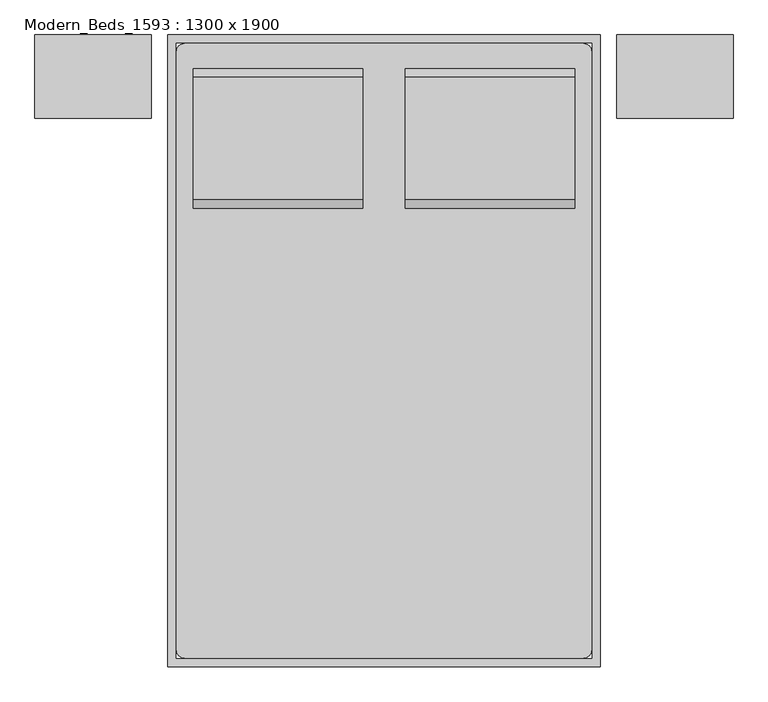
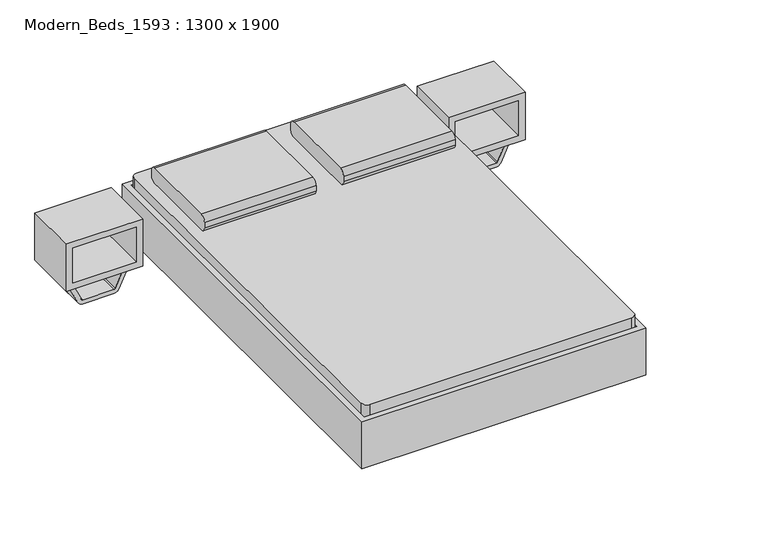
"""IFC4 building model written with IfcOpenShell, lengths in millimetres: furniture geometry, Modern_Beds_1593 : 1300 x 1900."""

from ifc_helpers import new_model, si_unit, point, frame, frame_2d, origin, place, context, project, spatial, polyline, circle_curve, trimmed, segment, composite_curve, outline, extrude, source, transform, mapped, element, save
from ifc_brep_helpers import plane_surface, cylinder_surface, revolved_surface, advanced_brep


def modern_beds_1593_1300_x_1900_cc95cf5d(model_context):
    return source(origin(), model_context, "Body", "SolidModel", [
        advanced_brep(
        [(-285.447541, -879.6295082, 196.85), (-285.447541, -879.6295082, 177.8), (-285.447541, -955.8295082, 177.8), (-285.447541, -955.8295082, 196.85), (-222.5113525, -879.6295082, 196.85), (-234.647541, -879.6295082, 177.8), (-234.647541, -955.8295082, 177.8), (-222.5113525, -955.8295082, 196.85), (-141.3115092, -879.6295082, 22.716374), (-158.5766725, -879.6295082, 14.6654962), (-158.5766725, -955.8295082, 14.6654962), (-141.3115092, -955.8295082, 22.716374), (-135.5564547, -879.6295082, 0.0), (-135.5564547, -879.6295082, 19.05), (-135.5564547, -955.8295082, 0.0), (-135.5564547, -955.8295082, 19.05), (-56.9439489, -879.6295082, 19.05), (-56.9439489, -879.6295082, 0.0), (-56.9439489, -955.8295082, 0.0), (-56.9439489, -955.8295082, 19.05), (-44.2439489, -879.6295082, 3.4029547), (-53.7689489, -879.6295082, 19.9007387), (-44.2439489, -955.8295082, 3.4029547), (-53.7689489, -955.8295082, 19.9007387), (10.7486643, -879.6295082, 57.15), (15.8530964, -879.6295082, 38.1), (15.8530964, -955.8295082, 38.1), (10.7486643, -955.8295082, 57.15), (667.5562537, -879.6295082, 57.15), (662.4518216, -879.6295082, 38.1), (662.4518216, -955.8295082, 38.1), (667.5562537, -955.8295082, 57.15), (732.0738669, -879.6295082, 19.9007387), (722.5488669, -879.6295082, 3.4029547), (722.5488669, -955.8295082, 3.4029547), (732.0738669, -955.8295082, 19.9007387), (735.2488669, -879.6295082, 0.0), (735.2488669, -879.6295082, 19.05), (735.2488669, -955.8295082, 0.0), (735.2488669, -955.8295082, 19.05), (813.8613728, -879.6295082, 19.05), (813.8613728, -879.6295082, 0.0), (813.8613728, -955.8295082, 0.0), (813.8613728, -955.8295082, 19.05), (836.8815906, -879.6295082, 14.6654962), (819.6164272, -879.6295082, 22.716374), (836.8815906, -955.8295082, 14.6654962), (819.6164272, -955.8295082, 22.716374), (900.8162705, -879.6295082, 196.85), (912.952459, -879.6295082, 177.8), (912.952459, -955.8295082, 177.8), (900.8162705, -955.8295082, 196.85), (963.752459, -879.6295082, 196.85), (963.752459, -955.8295082, 196.85), (963.752459, -955.8295082, 177.8), (963.752459, -879.6295082, 177.8)],
        [
            (0, 1),
            (1, 2),
            (2, 3),
            (3, 0),
            (0, 4),
            (4, 5),
            (5, 1),
            (5, 6),
            (6, 2),
            (6, 7),
            (7, 3),
            (7, 4),
            (4, 8),
            (8, 9),
            (9, 5),
            (9, 10),
            (10, 6),
            (10, 11),
            (11, 7),
            (11, 8),
            (12, 9, circle_curve(frame((-135.5564547, -879.6295082, 25.4), z_axis=(0.0, 1.0, 0.0), x_axis=(-0.9063077870366716, 0.0, -0.422618261740653)), 25.4)),
            (8, 13, circle_curve(frame((-135.5564547, -879.6295082, 25.4), z_axis=(0.0, -1.0, 0.0), x_axis=(-0.9063077870366716, 0.0, -0.422618261740653)), 6.35)),
            (13, 12),
            (14, 10, circle_curve(frame((-135.5564547, -955.8295082, 25.4), z_axis=(0.0, 1.0, 0.0), x_axis=(-0.9063077870366716, 0.0, -0.422618261740653)), 25.4)),
            (12, 14),
            (15, 11, circle_curve(frame((-135.5564547, -955.8295082, 25.4), z_axis=(0.0, 1.0, 0.0), x_axis=(-0.9063077870366716, 0.0, -0.422618261740653)), 6.35)),
            (14, 15),
            (15, 13),
            (13, 16),
            (16, 17),
            (17, 12),
            (17, 18),
            (18, 14),
            (18, 19),
            (19, 15),
            (19, 16),
            (20, 17, circle_curve(frame((-56.9439489, -879.6295082, 25.4), z_axis=(0.0, 1.0, 0.0), x_axis=(0.0, 0.0, -1.0)), 25.4)),
            (16, 21, circle_curve(frame((-56.9439489, -879.6295082, 25.4), z_axis=(0.0, -1.0, 0.0), x_axis=(0.0, 0.0, -1.0)), 6.35)),
            (21, 20),
            (22, 18, circle_curve(frame((-56.9439489, -955.8295082, 25.4), z_axis=(0.0, 1.0, 0.0), x_axis=(0.0, 0.0, -1.0)), 25.4)),
            (20, 22),
            (23, 19, circle_curve(frame((-56.9439489, -955.8295082, 25.4), z_axis=(0.0, 1.0, 0.0), x_axis=(0.0, 0.0, -1.0)), 6.35)),
            (22, 23),
            (23, 21),
            (21, 24),
            (24, 25),
            (25, 20),
            (25, 26),
            (26, 22),
            (26, 27),
            (27, 23),
            (27, 24),
            (24, 28),
            (28, 29),
            (29, 25),
            (29, 30),
            (30, 26),
            (30, 31),
            (31, 27),
            (31, 28),
            (28, 32),
            (32, 33),
            (33, 29),
            (33, 34),
            (34, 30),
            (34, 35),
            (35, 31),
            (35, 32),
            (36, 33, circle_curve(frame((735.2488669, -879.6295082, 25.4), z_axis=(0.0, 1.0, 0.0), x_axis=(-0.5000000000000527, 0.0, -0.8660254037844082)), 25.4)),
            (32, 37, circle_curve(frame((735.2488669, -879.6295082, 25.4), z_axis=(0.0, -1.0, 0.0), x_axis=(-0.5000000000000527, 0.0, -0.8660254037844082)), 6.35)),
            (37, 36),
            (38, 34, circle_curve(frame((735.2488669, -955.8295082, 25.4), z_axis=(0.0, 1.0, 0.0), x_axis=(-0.5000000000000527, 0.0, -0.8660254037844082)), 25.4)),
            (36, 38),
            (39, 35, circle_curve(frame((735.2488669, -955.8295082, 25.4), z_axis=(0.0, 1.0, 0.0), x_axis=(-0.5000000000000527, 0.0, -0.8660254037844082)), 6.35)),
            (38, 39),
            (39, 37),
            (37, 40),
            (40, 41),
            (41, 36),
            (41, 42),
            (42, 38),
            (42, 43),
            (43, 39),
            (43, 40),
            (44, 41, circle_curve(frame((813.8613728, -879.6295082, 25.4), z_axis=(0.0, 1.0, 0.0), x_axis=(0.0, 0.0, -1.0)), 25.4)),
            (40, 45, circle_curve(frame((813.8613728, -879.6295082, 25.4), z_axis=(0.0, -1.0, 0.0), x_axis=(0.0, 0.0, -1.0)), 6.35)),
            (45, 44),
            (46, 42, circle_curve(frame((813.8613728, -955.8295082, 25.4), z_axis=(0.0, 1.0, 0.0), x_axis=(0.0, 0.0, -1.0)), 25.4)),
            (44, 46),
            (47, 43, circle_curve(frame((813.8613728, -955.8295082, 25.4), z_axis=(0.0, 1.0, 0.0), x_axis=(0.0, 0.0, -1.0)), 6.35)),
            (46, 47),
            (47, 45),
            (45, 48),
            (48, 49),
            (49, 44),
            (49, 50),
            (50, 46),
            (50, 51),
            (51, 47),
            (51, 48),
            (52, 53),
            (53, 54),
            (54, 55),
            (55, 52),
            (48, 52),
            (55, 49),
            (54, 50),
            (53, 51),
        ],
        [
            plane_surface(frame((-285.447541, -1184.4295082, -127.5947323), z_axis=(-1.0, 0.0, 0.0), x_axis=(0.0, 1.0, 0.0))),
            plane_surface(frame((-285.447541, -879.6295082, 196.85), z_axis=(0.0, 1.0, 0.0), x_axis=(1.0, 0.0, 0.0))),
            plane_surface(frame((-285.447541, -879.6295082, 177.8), z_axis=(0.0, 0.0, -1.0), x_axis=(1.0, 0.0, 0.0))),
            plane_surface(frame((-285.447541, -955.8295082, 177.8), z_axis=(0.0, -1.0, 0.0), x_axis=(1.0, 0.0, 0.0))),
            plane_surface(frame((-285.447541, -955.8295082, 196.85), z_axis=(0.0, 0.0, 1.0), x_axis=(1.0, 0.0, 0.0))),
            plane_surface(frame((-222.5113525, -879.6295082, 196.85), z_axis=(0.0, 1.0, 0.0), x_axis=(0.4226182617406711, 0.0, -0.9063077870366633))),
            plane_surface(frame((-234.647541, -879.6295082, 177.8), z_axis=(-0.9063077870366631, 0.0, -0.4226182617406711), x_axis=(0.4226182617406711, 0.0, -0.9063077870366631))),
            plane_surface(frame((-234.647541, -955.8295082, 177.8), z_axis=(0.0, -1.0, 0.0), x_axis=(0.4226182617406708, 0.0, -0.9063077870366634))),
            plane_surface(frame((-222.5113525, -955.8295082, 196.85), z_axis=(0.9063077870366631, 0.0, 0.4226182617406713), x_axis=(0.4226182617406713, 0.0, -0.9063077870366631))),
            plane_surface(frame((-135.5564547, -879.6295082, 25.4), z_axis=(0.0, 1.0000000000000002, 0.0), x_axis=(-0.9063077870366717, 0.0, -0.42261826174065303))),
            cylinder_surface(frame((-135.5564547, -1184.4295082, 25.4), z_axis=(0.0, -1.0, 0.0), x_axis=(-0.9063077870366716, 0.0, -0.422618261740653)), 25.4),
            plane_surface(frame((-135.5564547, -955.8295082, 25.4), z_axis=(0.0, -1.0000000000000002, 0.0), x_axis=(-0.9063077870366717, 0.0, -0.42261826174065303))),
            revolved_surface(polyline([(-141.31150914768284, -955.8295082, 22.716374037946853), (-141.31150914768284, -879.6295082, 22.716374037946853)]), (-135.5564547, -1184.4295082, 25.4), (0.0, -1.0, 0.0)),
            plane_surface(frame((-135.5564547, -879.6295082, 19.05), z_axis=(0.0, 1.0, 0.0), x_axis=(1.0, 0.0, 0.0))),
            plane_surface(frame((-135.5564547, -879.6295082, 0.0), z_axis=(0.0, 0.0, -1.0), x_axis=(1.0, 0.0, 0.0))),
            plane_surface(frame((-135.5564547, -955.8295082, 0.0), z_axis=(0.0, -1.0, 0.0), x_axis=(1.0, 0.0, 0.0))),
            plane_surface(frame((-135.5564547, -955.8295082, 19.05), z_axis=(0.0, 0.0, 1.0), x_axis=(1.0, 0.0, 0.0))),
            plane_surface(frame((-56.9439489, -879.6295082, 25.4), z_axis=(0.0, 1.0, 0.0), x_axis=(0.0, 0.0, -1.0))),
            cylinder_surface(frame((-56.9439489, -1184.4295082, 25.4), z_axis=(0.0, -1.0, 0.0), x_axis=(0.0, 0.0, -1.0)), 25.4),
            plane_surface(frame((-56.9439489, -955.8295082, 25.4), z_axis=(0.0, -1.0, 0.0), x_axis=(0.0, 0.0, -1.0))),
            revolved_surface(polyline([(-56.9439489, -955.8295082, 19.049999999999997), (-56.9439489, -879.6295082, 19.049999999999997)]), (-56.9439489, -1184.4295082, 25.4), (0.0, -1.0, 0.0)),
            plane_surface(frame((-53.7689489, -879.6295082, 19.9007387), z_axis=(0.0, 1.0, 0.0), x_axis=(0.8660254037844797, 0.0, 0.4999999999999289))),
            plane_surface(frame((-44.2439489, -879.6295082, 3.4029547), z_axis=(0.49999999999992967, 0.0, -0.8660254037844792), x_axis=(0.8660254037844792, 0.0, 0.49999999999992967))),
            plane_surface(frame((-44.2439489, -955.8295082, 3.4029547), z_axis=(0.0, -1.0, 0.0), x_axis=(0.8660254037844796, 0.0, 0.4999999999999291))),
            plane_surface(frame((-53.7689489, -955.8295082, 19.9007387), z_axis=(-0.4999999999999289, 0.0, 0.8660254037844798), x_axis=(0.8660254037844798, 0.0, 0.4999999999999289))),
            plane_surface(frame((10.7486643, -879.6295082, 57.15), z_axis=(0.0, 1.0, 0.0), x_axis=(1.0, 0.0, 0.0))),
            plane_surface(frame((15.8530964, -879.6295082, 38.1), z_axis=(0.0, 0.0, -1.0), x_axis=(1.0, 0.0, 0.0))),
            plane_surface(frame((15.8530964, -955.8295082, 38.1), z_axis=(0.0, -1.0, 0.0), x_axis=(1.0, 0.0, 0.0))),
            plane_surface(frame((10.7486643, -955.8295082, 57.15), z_axis=(0.0, 0.0, 1.0), x_axis=(1.0, 0.0, 0.0))),
            plane_surface(frame((667.5562537, -879.6295082, 57.15), z_axis=(0.0, 1.0, 0.0), x_axis=(0.86602540378441, 0.0, -0.5000000000000497))),
            plane_surface(frame((662.4518216, -879.6295082, 38.1), z_axis=(-0.5000000000000513, 0.0, -0.8660254037844091), x_axis=(0.8660254037844091, 0.0, -0.5000000000000513))),
            plane_surface(frame((662.4518216, -955.8295082, 38.1), z_axis=(0.0, -1.0000000000000002, 0.0), x_axis=(0.866025403784409, 0.0, -0.5000000000000516))),
            plane_surface(frame((667.5562537, -955.8295082, 57.15), z_axis=(0.5000000000000515, 0.0, 0.866025403784409), x_axis=(0.866025403784409, 0.0, -0.5000000000000515))),
            plane_surface(frame((735.2488669, -879.6295082, 25.4), z_axis=(0.0, 1.0, 0.0), x_axis=(-0.5000000000000527, 0.0, -0.8660254037844082))),
            cylinder_surface(frame((735.2488669, -1184.4295082, 25.4), z_axis=(0.0, -1.0, 0.0), x_axis=(-0.5000000000000527, 0.0, -0.8660254037844082)), 25.4),
            plane_surface(frame((735.2488669, -955.8295082, 25.4), z_axis=(0.0, -1.0, 0.0), x_axis=(-0.5000000000000527, 0.0, -0.8660254037844082))),
            revolved_surface(polyline([(732.0738668999998, -955.8295082, 19.900738685969007), (732.0738668999998, -879.6295082, 19.900738685969007)]), (735.2488669, -1184.4295082, 25.4), (0.0, -1.0, 0.0)),
            plane_surface(frame((735.2488669, -879.6295082, 19.05), z_axis=(0.0, 1.0, 0.0), x_axis=(1.0, 0.0, 0.0))),
            plane_surface(frame((735.2488669, -879.6295082, 0.0), z_axis=(0.0, 0.0, -1.0), x_axis=(1.0, 0.0, 0.0))),
            plane_surface(frame((735.2488669, -955.8295082, 0.0), z_axis=(0.0, -1.0, 0.0), x_axis=(1.0, 0.0, 0.0))),
            plane_surface(frame((735.2488669, -955.8295082, 19.05), z_axis=(0.0, 0.0, 1.0), x_axis=(1.0, 0.0, 0.0))),
            plane_surface(frame((813.8613728, -879.6295082, 25.4), z_axis=(0.0, 1.0, 0.0), x_axis=(0.0, 0.0, -1.0))),
            cylinder_surface(frame((813.8613728, -1184.4295082, 25.4), z_axis=(0.0, -1.0, 0.0), x_axis=(0.0, 0.0, -1.0)), 25.4),
            plane_surface(frame((813.8613728, -955.8295082, 25.4), z_axis=(0.0, -1.0, 0.0), x_axis=(0.0, 0.0, -1.0))),
            revolved_surface(polyline([(813.8613728, -955.8295082, 19.049999999999997), (813.8613728, -879.6295082, 19.049999999999997)]), (813.8613728, -1184.4295082, 25.4), (0.0, -1.0, 0.0)),
            plane_surface(frame((819.6164272, -879.6295082, 22.716374), z_axis=(0.0, 1.0, 0.0), x_axis=(0.42261826174054257, 0.0, 0.9063077870367231))),
            plane_surface(frame((836.8815906, -879.6295082, 14.6654962), z_axis=(0.9063077870367228, 0.0, -0.42261826174054334), x_axis=(0.42261826174054334, 0.0, 0.9063077870367228))),
            plane_surface(frame((836.8815906, -955.8295082, 14.6654962), z_axis=(0.0, -1.0000000000000002, 0.0), x_axis=(0.42261826174054296, 0.0, 0.906307787036723))),
            plane_surface(frame((819.6164272, -955.8295082, 22.716374), z_axis=(-0.9063077870367229, 0.0, 0.42261826174054307), x_axis=(0.42261826174054307, 0.0, 0.9063077870367229))),
            plane_surface(frame((963.752459, -1184.4295082, -127.5947323), z_axis=(1.0, 0.0, 0.0), x_axis=(0.0, 1.0, 0.0))),
            plane_surface(frame((900.8162705, -879.6295082, 196.85), z_axis=(0.0, 1.0, 0.0), x_axis=(1.0, 0.0, 0.0))),
            plane_surface(frame((912.952459, -879.6295082, 177.8), z_axis=(0.0, 0.0, -1.0), x_axis=(1.0, 0.0, 0.0))),
            plane_surface(frame((912.952459, -955.8295082, 177.8), z_axis=(0.0, -1.0, 0.0), x_axis=(1.0, 0.0, 0.0))),
            plane_surface(frame((900.8162705, -955.8295082, 196.85), z_axis=(0.0, 0.0, 1.0), x_axis=(1.0, 0.0, 0.0))),
        ],
        [
            (0, [[1, 2, 3, 4]]),
            (1, [[-1, 5, 6, 7]]),
            (2, [[-2, -7, 8, 9]]),
            (3, [[-3, -9, 10, 11]]),
            (4, [[-4, -11, 12, -5]]),
            (5, [[-6, 13, 14, 15]]),
            (6, [[-8, -15, 16, 17]]),
            (7, [[-10, -17, 18, 19]]),
            (8, [[-12, -19, 20, -13]]),
            (9, [[21, -14, 22, 23]]),
            (10, [[24, -16, -21, 25]]),
            (11, [[26, -18, -24, 27]]),
            (12, [[-22, -20, -26, 28]]),
            (13, [[-23, 29, 30, 31]]),
            (14, [[-25, -31, 32, 33]]),
            (15, [[-27, -33, 34, 35]]),
            (16, [[-28, -35, 36, -29]]),
            (17, [[37, -30, 38, 39]]),
            (18, [[40, -32, -37, 41]]),
            (19, [[42, -34, -40, 43]]),
            (20, [[-38, -36, -42, 44]]),
            (21, [[-39, 45, 46, 47]]),
            (22, [[-41, -47, 48, 49]]),
            (23, [[-43, -49, 50, 51]]),
            (24, [[-44, -51, 52, -45]]),
            (25, [[-46, 53, 54, 55]]),
            (26, [[-48, -55, 56, 57]]),
            (27, [[-50, -57, 58, 59]]),
            (28, [[-52, -59, 60, -53]]),
            (29, [[-54, 61, 62, 63]]),
            (30, [[-56, -63, 64, 65]]),
            (31, [[-58, -65, 66, 67]]),
            (32, [[-60, -67, 68, -61]]),
            (33, [[69, -62, 70, 71]]),
            (34, [[72, -64, -69, 73]]),
            (35, [[74, -66, -72, 75]]),
            (36, [[-70, -68, -74, 76]]),
            (37, [[-71, 77, 78, 79]]),
            (38, [[-73, -79, 80, 81]]),
            (39, [[-75, -81, 82, 83]]),
            (40, [[-76, -83, 84, -77]]),
            (41, [[85, -78, 86, 87]]),
            (42, [[88, -80, -85, 89]]),
            (43, [[90, -82, -88, 91]]),
            (44, [[-86, -84, -90, 92]]),
            (45, [[-87, 93, 94, 95]]),
            (46, [[-89, -95, 96, 97]]),
            (47, [[-91, -97, 98, 99]]),
            (48, [[-92, -99, 100, -93]]),
            (49, [[101, 102, 103, 104]]),
            (50, [[-94, 105, -104, 106]]),
            (51, [[-96, -106, -103, 107]]),
            (52, [[-98, -107, -102, 108]]),
            (53, [[-100, -108, -101, -105]]),
        ],
    ),
        advanced_brep(
        [(-285.1231784, 461.5704918, 177.8), (-285.1231784, 385.3704918, 177.8), (-285.1231784, 385.3704918, 196.85), (-285.1231784, 461.5704918, 196.85), (-234.3231784, 461.5704918, 177.8), (-234.3231784, 385.3704918, 177.8), (-222.1869899, 385.3704918, 196.85), (-222.1869899, 461.5704918, 196.85), (-158.2523099, 461.5704918, 14.6654962), (-158.2523099, 385.3704918, 14.6654962), (-140.9871466, 385.3704918, 22.716374), (-140.9871466, 461.5704918, 22.716374), (-135.2320921, 385.3704918, 0.0), (-135.2320921, 461.5704918, 0.0), (-135.2320921, 385.3704918, 19.05), (-135.2320921, 461.5704918, 19.05), (-56.6195862, 461.5704918, 0.0), (-56.6195862, 385.3704918, 0.0), (-56.6195862, 385.3704918, 19.05), (-56.6195862, 461.5704918, 19.05), (-43.9195862, 385.3704918, 3.4029547), (-43.9195862, 461.5704918, 3.4029547), (-53.4445862, 385.3704918, 19.9007387), (-53.4445862, 461.5704918, 19.9007387), (16.177459, 461.5704918, 38.1), (16.177459, 385.3704918, 38.1), (11.0730269, 385.3704918, 57.15), (11.0730269, 461.5704918, 57.15), (662.4518216, 461.5704918, 38.1), (662.4518216, 385.3704918, 38.1), (667.5562537, 385.3704918, 57.15), (667.5562537, 461.5704918, 57.15), (722.5488669, 461.5704918, 3.4029547), (722.5488669, 385.3704918, 3.4029547), (732.0738669, 385.3704918, 19.9007387), (732.0738669, 461.5704918, 19.9007387), (735.2488669, 385.3704918, 0.0), (735.2488669, 461.5704918, 0.0), (735.2488669, 385.3704918, 19.05), (735.2488669, 461.5704918, 19.05), (813.8613728, 461.5704918, 0.0), (813.8613728, 385.3704918, 0.0), (813.8613728, 385.3704918, 19.05), (813.8613728, 461.5704918, 19.05), (836.8815906, 385.3704918, 14.6654962), (836.8815906, 461.5704918, 14.6654962), (819.6164272, 385.3704918, 22.716374), (819.6164272, 461.5704918, 22.716374), (912.952459, 461.5704918, 177.8), (912.952459, 385.3704918, 177.8), (900.8162705, 385.3704918, 196.85), (900.8162705, 461.5704918, 196.85), (963.752459, 461.5704918, 177.8), (963.752459, 461.5704918, 196.85), (963.752459, 385.3704918, 196.85), (963.752459, 385.3704918, 177.8)],
        [
            (0, 1),
            (1, 2),
            (2, 3),
            (3, 0),
            (0, 4),
            (4, 5),
            (5, 1),
            (5, 6),
            (6, 2),
            (6, 7),
            (7, 3),
            (7, 4),
            (4, 8),
            (8, 9),
            (9, 5),
            (9, 10),
            (10, 6),
            (10, 11),
            (11, 7),
            (11, 8),
            (12, 9, circle_curve(frame((-135.2320921, 385.3704918, 25.4), z_axis=(0.0, 1.0, 0.0), x_axis=(-0.9063077870366478, 0.0, -0.4226182617407041)), 25.4)),
            (8, 13, circle_curve(frame((-135.2320921, 461.5704918, 25.4), z_axis=(0.0, -1.0, 0.0), x_axis=(-0.9063077870366478, 0.0, -0.4226182617407041)), 25.4)),
            (13, 12),
            (14, 10, circle_curve(frame((-135.2320921, 385.3704918, 25.4), z_axis=(0.0, 1.0, 0.0), x_axis=(-0.9063077870366478, 0.0, -0.4226182617407041)), 6.35)),
            (12, 14),
            (15, 11, circle_curve(frame((-135.2320921, 461.5704918, 25.4), z_axis=(0.0, 1.0, 0.0), x_axis=(-0.9063077870366478, 0.0, -0.4226182617407041)), 6.35)),
            (14, 15),
            (15, 13),
            (13, 16),
            (16, 17),
            (17, 12),
            (17, 18),
            (18, 14),
            (18, 19),
            (19, 15),
            (19, 16),
            (20, 17, circle_curve(frame((-56.6195862, 385.3704918, 25.4), z_axis=(0.0, 1.0, 0.0), x_axis=(0.0, 0.0, -1.0)), 25.4)),
            (16, 21, circle_curve(frame((-56.6195862, 461.5704918, 25.4), z_axis=(0.0, -1.0, 0.0), x_axis=(0.0, 0.0, -1.0)), 25.4)),
            (21, 20),
            (22, 18, circle_curve(frame((-56.6195862, 385.3704918, 25.4), z_axis=(0.0, 1.0, 0.0), x_axis=(0.0, 0.0, -1.0)), 6.35)),
            (20, 22),
            (23, 19, circle_curve(frame((-56.6195862, 461.5704918, 25.4), z_axis=(0.0, 1.0, 0.0), x_axis=(0.0, 0.0, -1.0)), 6.35)),
            (22, 23),
            (23, 21),
            (21, 24),
            (24, 25),
            (25, 20),
            (25, 26),
            (26, 22),
            (26, 27),
            (27, 23),
            (27, 24),
            (24, 28),
            (28, 29),
            (29, 25),
            (29, 30),
            (30, 26),
            (30, 31),
            (31, 27),
            (31, 28),
            (28, 32),
            (32, 33),
            (33, 29),
            (33, 34),
            (34, 30),
            (34, 35),
            (35, 31),
            (35, 32),
            (36, 33, circle_curve(frame((735.2488669, 385.3704918, 25.4), z_axis=(0.0, 1.0, 0.0), x_axis=(-0.5000000000000581, 0.0, -0.8660254037844051)), 25.4)),
            (32, 37, circle_curve(frame((735.2488669, 461.5704918, 25.4), z_axis=(0.0, -1.0, 0.0), x_axis=(-0.5000000000000581, 0.0, -0.8660254037844051)), 25.4)),
            (37, 36),
            (38, 34, circle_curve(frame((735.2488669, 385.3704918, 25.4), z_axis=(0.0, 1.0, 0.0), x_axis=(-0.5000000000000581, 0.0, -0.8660254037844051)), 6.35)),
            (36, 38),
            (39, 35, circle_curve(frame((735.2488669, 461.5704918, 25.4), z_axis=(0.0, 1.0, 0.0), x_axis=(-0.5000000000000581, 0.0, -0.8660254037844051)), 6.35)),
            (38, 39),
            (39, 37),
            (37, 40),
            (40, 41),
            (41, 36),
            (41, 42),
            (42, 38),
            (42, 43),
            (43, 39),
            (43, 40),
            (44, 41, circle_curve(frame((813.8613728, 385.3704918, 25.4), z_axis=(0.0, 1.0, 0.0), x_axis=(0.0, 0.0, -1.0)), 25.4)),
            (40, 45, circle_curve(frame((813.8613728, 461.5704918, 25.4), z_axis=(0.0, -1.0, 0.0), x_axis=(0.0, 0.0, -1.0)), 25.4)),
            (45, 44),
            (46, 42, circle_curve(frame((813.8613728, 385.3704918, 25.4), z_axis=(0.0, 1.0, 0.0), x_axis=(0.0, 0.0, -1.0)), 6.35)),
            (44, 46),
            (47, 43, circle_curve(frame((813.8613728, 461.5704918, 25.4), z_axis=(0.0, 1.0, 0.0), x_axis=(0.0, 0.0, -1.0)), 6.35)),
            (46, 47),
            (47, 45),
            (45, 48),
            (48, 49),
            (49, 44),
            (49, 50),
            (50, 46),
            (50, 51),
            (51, 47),
            (51, 48),
            (52, 53),
            (53, 54),
            (54, 55),
            (55, 52),
            (48, 52),
            (55, 49),
            (54, 50),
            (53, 51),
        ],
        [
            plane_surface(frame((-285.1231784, 715.5704918, -152.9490627), z_axis=(-1.0, 0.0, 0.0), x_axis=(0.0, 1.0, 0.0))),
            plane_surface(frame((-285.1231784, 461.5704918, 177.8), z_axis=(0.0, 0.0, -1.0), x_axis=(1.0, 0.0, 0.0))),
            plane_surface(frame((-285.1231784, 385.3704918, 177.8), z_axis=(0.0, -1.0, 0.0), x_axis=(1.0, 0.0, 0.0))),
            plane_surface(frame((-285.1231784, 385.3704918, 196.85), z_axis=(0.0, 0.0, 1.0), x_axis=(1.0, 0.0, 0.0))),
            plane_surface(frame((-285.1231784, 461.5704918, 196.85), z_axis=(0.0, 1.0, 0.0), x_axis=(1.0, 0.0, 0.0))),
            plane_surface(frame((-234.3231784, 461.5704918, 177.8), z_axis=(-0.9063077870366485, 0.0, -0.42261826174070266), x_axis=(0.42261826174070266, 0.0, -0.9063077870366485))),
            plane_surface(frame((-234.3231784, 385.3704918, 177.8), z_axis=(0.0, -1.0, 0.0), x_axis=(0.4226182617407026, 0.0, -0.9063077870366485))),
            plane_surface(frame((-222.1869899, 385.3704918, 196.85), z_axis=(0.9063077870366485, 0.0, 0.42261826174070266), x_axis=(0.42261826174070266, 0.0, -0.9063077870366485))),
            plane_surface(frame((-222.1869899, 461.5704918, 196.85), z_axis=(0.0, 1.0000000000000002, 0.0), x_axis=(0.4226182617407026, 0.0, -0.9063077870366486))),
            cylinder_surface(frame((-135.2320921, 715.5704918, 25.4), z_axis=(0.0, -1.0, 0.0), x_axis=(-0.9063077870366478, 0.0, -0.4226182617407041)), 25.4),
            plane_surface(frame((-135.2320921, 385.3704918, 25.4), z_axis=(0.0, -1.0, 0.0), x_axis=(-0.9063077870366478, 0.0, -0.4226182617407041))),
            revolved_surface(polyline([(-140.9871465476827, 385.3704918, 22.71637403794653), (-140.9871465476827, 461.5704918, 22.71637403794653)]), (-135.2320921, 715.5704918, 25.4), (0.0, -1.0, 0.0)),
            plane_surface(frame((-135.2320921, 461.5704918, 25.4), z_axis=(0.0, 1.0, 0.0), x_axis=(-0.9063077870366478, 0.0, -0.4226182617407041))),
            plane_surface(frame((-135.2320921, 461.5704918, 0.0), z_axis=(0.0, 0.0, -1.0), x_axis=(1.0, 0.0, 0.0))),
            plane_surface(frame((-135.2320921, 385.3704918, 0.0), z_axis=(0.0, -1.0, 0.0), x_axis=(1.0, 0.0, 0.0))),
            plane_surface(frame((-135.2320921, 385.3704918, 19.05), z_axis=(0.0, 0.0, 1.0), x_axis=(1.0, 0.0, 0.0))),
            plane_surface(frame((-135.2320921, 461.5704918, 19.05), z_axis=(0.0, 1.0, 0.0), x_axis=(1.0, 0.0, 0.0))),
            cylinder_surface(frame((-56.6195862, 715.5704918, 25.4), z_axis=(0.0, -1.0, 0.0), x_axis=(0.0, 0.0, -1.0)), 25.4),
            plane_surface(frame((-56.6195862, 385.3704918, 25.4), z_axis=(0.0, -1.0, 0.0), x_axis=(0.0, 0.0, -1.0))),
            revolved_surface(polyline([(-56.6195862, 385.3704918, 19.049999999999997), (-56.6195862, 461.5704918, 19.049999999999997)]), (-56.6195862, 715.5704918, 25.4), (0.0, -1.0, 0.0)),
            plane_surface(frame((-56.6195862, 461.5704918, 25.4), z_axis=(0.0, 1.0, 0.0), x_axis=(0.0, 0.0, -1.0))),
            plane_surface(frame((-43.9195862, 461.5704918, 3.4029547), z_axis=(0.4999999999998787, 0.0, -0.8660254037845087), x_axis=(0.8660254037845087, 0.0, 0.4999999999998787))),
            plane_surface(frame((-43.9195862, 385.3704918, 3.4029547), z_axis=(0.0, -1.0, 0.0), x_axis=(0.8660254037845089, 0.0, 0.4999999999998783))),
            plane_surface(frame((-53.4445862, 385.3704918, 19.9007387), z_axis=(-0.49999999999987854, 0.0, 0.8660254037845088), x_axis=(0.8660254037845088, 0.0, 0.49999999999987854))),
            plane_surface(frame((-53.4445862, 461.5704918, 19.9007387), z_axis=(0.0, 1.0, 0.0), x_axis=(0.8660254037845092, 0.0, 0.4999999999998779))),
            plane_surface(frame((16.177459, 461.5704918, 38.1), z_axis=(0.0, 0.0, -1.0), x_axis=(1.0, 0.0, 0.0))),
            plane_surface(frame((16.177459, 385.3704918, 38.1), z_axis=(0.0, -1.0, 0.0), x_axis=(1.0, 0.0, 0.0))),
            plane_surface(frame((11.0730269, 385.3704918, 57.15), z_axis=(0.0, 0.0, 1.0), x_axis=(1.0, 0.0, 0.0))),
            plane_surface(frame((11.0730269, 461.5704918, 57.15), z_axis=(0.0, 1.0, 0.0), x_axis=(1.0, 0.0, 0.0))),
            plane_surface(frame((662.4518216, 461.5704918, 38.1), z_axis=(-0.5000000000000503, 0.0, -0.8660254037844097), x_axis=(0.8660254037844097, 0.0, -0.5000000000000503))),
            plane_surface(frame((662.4518216, 385.3704918, 38.1), z_axis=(0.0, -1.0000000000000002, 0.0), x_axis=(0.8660254037844094, 0.0, -0.5000000000000508))),
            plane_surface(frame((667.5562537, 385.3704918, 57.15), z_axis=(0.5000000000000506, 0.0, 0.8660254037844094), x_axis=(0.8660254037844094, 0.0, -0.5000000000000506))),
            plane_surface(frame((667.5562537, 461.5704918, 57.15), z_axis=(0.0, 1.0, 0.0), x_axis=(0.8660254037844094, 0.0, -0.5000000000000506))),
            cylinder_surface(frame((735.2488669, 715.5704918, 25.4), z_axis=(0.0, -1.0, 0.0), x_axis=(-0.5000000000000581, 0.0, -0.8660254037844051)), 25.4),
            plane_surface(frame((735.2488669, 385.3704918, 25.4), z_axis=(0.0, -1.0000000000000002, 0.0), x_axis=(-0.5000000000000582, 0.0, -0.8660254037844052))),
            revolved_surface(polyline([(732.0738668999996, 385.3704918, 19.900738685969028), (732.0738668999996, 461.5704918, 19.900738685969028)]), (735.2488669, 715.5704918, 25.4), (0.0, -1.0, 0.0)),
            plane_surface(frame((735.2488669, 461.5704918, 25.4), z_axis=(0.0, 1.0000000000000002, 0.0), x_axis=(-0.5000000000000582, 0.0, -0.8660254037844052))),
            plane_surface(frame((735.2488669, 461.5704918, 0.0), z_axis=(0.0, 0.0, -1.0), x_axis=(1.0, 0.0, 0.0))),
            plane_surface(frame((735.2488669, 385.3704918, 0.0), z_axis=(0.0, -1.0, 0.0), x_axis=(1.0, 0.0, 0.0))),
            plane_surface(frame((735.2488669, 385.3704918, 19.05), z_axis=(0.0, 0.0, 1.0), x_axis=(1.0, 0.0, 0.0))),
            plane_surface(frame((735.2488669, 461.5704918, 19.05), z_axis=(0.0, 1.0, 0.0), x_axis=(1.0, 0.0, 0.0))),
            cylinder_surface(frame((813.8613728, 715.5704918, 25.4), z_axis=(0.0, -1.0, 0.0), x_axis=(0.0, 0.0, -1.0)), 25.4),
            plane_surface(frame((813.8613728, 385.3704918, 25.4), z_axis=(0.0, -1.0, 0.0), x_axis=(0.0, 0.0, -1.0))),
            revolved_surface(polyline([(813.8613728, 385.3704918, 19.049999999999997), (813.8613728, 461.5704918, 19.049999999999997)]), (813.8613728, 715.5704918, 25.4), (0.0, -1.0, 0.0)),
            plane_surface(frame((813.8613728, 461.5704918, 25.4), z_axis=(0.0, 1.0, 0.0), x_axis=(0.0, 0.0, -1.0))),
            plane_surface(frame((836.8815906, 461.5704918, 14.6654962), z_axis=(0.9063077870366775, 0.0, -0.4226182617406406), x_axis=(0.4226182617406406, 0.0, 0.9063077870366775))),
            plane_surface(frame((836.8815906, 385.3704918, 14.6654962), z_axis=(0.0, -1.0, 0.0), x_axis=(0.42261826174064043, 0.0, 0.9063077870366775))),
            plane_surface(frame((819.6164272, 385.3704918, 22.716374), z_axis=(-0.9063077870366779, 0.0, 0.4226182617406395), x_axis=(0.4226182617406395, 0.0, 0.9063077870366779))),
            plane_surface(frame((819.6164272, 461.5704918, 22.716374), z_axis=(0.0, 1.0, 0.0), x_axis=(0.42261826174064027, 0.0, 0.9063077870366776))),
            plane_surface(frame((963.752459, 715.5704918, -152.9490627), z_axis=(1.0, 0.0, 0.0), x_axis=(0.0, 1.0, 0.0))),
            plane_surface(frame((912.952459, 461.5704918, 177.8), z_axis=(0.0, 0.0, -1.0), x_axis=(1.0, 0.0, 0.0))),
            plane_surface(frame((912.952459, 385.3704918, 177.8), z_axis=(0.0, -1.0, 0.0), x_axis=(1.0, 0.0, 0.0))),
            plane_surface(frame((900.8162705, 385.3704918, 196.85), z_axis=(0.0, 0.0, 1.0), x_axis=(1.0, 0.0, 0.0))),
            plane_surface(frame((900.8162705, 461.5704918, 196.85), z_axis=(0.0, 1.0, 0.0), x_axis=(1.0, 0.0, 0.0))),
        ],
        [
            (0, [[1, 2, 3, 4]]),
            (1, [[-1, 5, 6, 7]]),
            (2, [[-2, -7, 8, 9]]),
            (3, [[-3, -9, 10, 11]]),
            (4, [[-4, -11, 12, -5]]),
            (5, [[-6, 13, 14, 15]]),
            (6, [[-8, -15, 16, 17]]),
            (7, [[-10, -17, 18, 19]]),
            (8, [[-12, -19, 20, -13]]),
            (9, [[21, -14, 22, 23]]),
            (10, [[24, -16, -21, 25]]),
            (11, [[26, -18, -24, 27]]),
            (12, [[-22, -20, -26, 28]]),
            (13, [[-23, 29, 30, 31]]),
            (14, [[-25, -31, 32, 33]]),
            (15, [[-27, -33, 34, 35]]),
            (16, [[-28, -35, 36, -29]]),
            (17, [[37, -30, 38, 39]]),
            (18, [[40, -32, -37, 41]]),
            (19, [[42, -34, -40, 43]]),
            (20, [[-38, -36, -42, 44]]),
            (21, [[-39, 45, 46, 47]]),
            (22, [[-41, -47, 48, 49]]),
            (23, [[-43, -49, 50, 51]]),
            (24, [[-44, -51, 52, -45]]),
            (25, [[-46, 53, 54, 55]]),
            (26, [[-48, -55, 56, 57]]),
            (27, [[-50, -57, 58, 59]]),
            (28, [[-52, -59, 60, -53]]),
            (29, [[-54, 61, 62, 63]]),
            (30, [[-56, -63, 64, 65]]),
            (31, [[-58, -65, 66, 67]]),
            (32, [[-60, -67, 68, -61]]),
            (33, [[69, -62, 70, 71]]),
            (34, [[72, -64, -69, 73]]),
            (35, [[74, -66, -72, 75]]),
            (36, [[-70, -68, -74, 76]]),
            (37, [[-71, 77, 78, 79]]),
            (38, [[-73, -79, 80, 81]]),
            (39, [[-75, -81, 82, 83]]),
            (40, [[-76, -83, 84, -77]]),
            (41, [[85, -78, 86, 87]]),
            (42, [[88, -80, -85, 89]]),
            (43, [[90, -82, -88, 91]]),
            (44, [[-86, -84, -90, 92]]),
            (45, [[-87, 93, 94, 95]]),
            (46, [[-89, -95, 96, 97]]),
            (47, [[-91, -97, 98, 99]]),
            (48, [[-92, -99, 100, -93]]),
            (49, [[101, 102, 103, 104]]),
            (50, [[-94, 105, -104, 106]]),
            (51, [[-96, -106, -103, 107]]),
            (52, [[-98, -107, -102, 108]]),
            (53, [[-100, -108, -101, -105]]),
        ],
    ),
        extrude(outline(composite_curve([segment(polyline([(-260.047541, 690.1704918), (938.352459, 690.1704918)]), True, "CONTINUOUS"), segment(trimmed(circle_curve(frame_2d((938.352459, 664.7704918)), 25.4), [point((938.352459, 690.1704918))], [point((963.752459, 664.7704918))], False, "CARTESIAN"), True, "CONTINUOUS"), segment(polyline([(963.752459, 664.7704918), (963.752459, -1133.6295082)]), True, "CONTINUOUS"), segment(trimmed(circle_curve(frame_2d((938.352459, -1133.6295082)), 25.4), [point((963.752459, -1133.6295082))], [point((938.352459, -1159.0295082))], False, "CARTESIAN"), True, "CONTINUOUS"), segment(polyline([(938.352459, -1159.0295082), (-260.047541, -1159.0295082)]), True, "CONTINUOUS"), segment(trimmed(circle_curve(frame_2d((-260.047541, -1133.6295082)), 25.4), [point((-260.047541, -1159.0295082))], [point((-285.447541, -1133.6295082))], False, "CARTESIAN"), True, "CONTINUOUS"), segment(polyline([(-285.447541, -1133.6295082), (-285.447541, 664.7704918)]), True, "CONTINUOUS"), segment(trimmed(circle_curve(frame_2d((-260.047541, 664.7704918)), 25.4), [point((-285.447541, 664.7704918))], [point((-260.047541, 690.1704918))], False, "CARTESIAN"), True, "CONTINUOUS")], self_intersect=False)), frame((0.0, 0.0, 203.2), z_axis=(0.0, 0.0, 1.0), x_axis=(1.0, 0.0, 0.0)), (0.0, 0.0, 1.0), 203.2),
        extrude(outline(composite_curve([segment(polyline([(588.5704918, 406.4), (220.2704918, 406.4)]), True, "CONTINUOUS"), segment(trimmed(circle_curve(frame_2d((220.2704918, 431.8)), 25.4), [point((220.2704918, 406.4))], [point((194.8704918, 431.8))], False, "CARTESIAN"), True, "CONTINUOUS"), segment(polyline([(194.8704918, 431.8), (194.8704918, 457.2)]), True, "CONTINUOUS"), segment(trimmed(circle_curve(frame_2d((220.2704918, 457.2)), 25.4), [point((194.8704918, 457.2))], [point((220.2704918, 482.6))], False, "CARTESIAN"), True, "CONTINUOUS"), segment(polyline([(220.2704918, 482.6), (588.5704918, 482.6)]), True, "CONTINUOUS"), segment(trimmed(circle_curve(frame_2d((588.5704918, 457.2)), 25.4), [point((588.5704918, 482.6))], [point((613.9704918, 457.2))], False, "CARTESIAN"), True, "CONTINUOUS"), segment(polyline([(613.9704918, 457.2), (613.9704918, 431.8)]), True, "CONTINUOUS"), segment(trimmed(circle_curve(frame_2d((588.5704918, 431.8)), 25.4), [point((613.9704918, 431.8))], [point((588.5704918, 406.4))], False, "CARTESIAN"), True, "CONTINUOUS")], self_intersect=False)), frame((-234.647541, 0.0, 0.0), z_axis=(1.0, 0.0, 0.0), x_axis=(0.0, 1.0, 0.0)), (0.0, 0.0, 1.0), 510.3),
        extrude(outline(composite_curve([segment(polyline([(588.5704918, 406.4), (220.2704918, 406.4)]), True, "CONTINUOUS"), segment(trimmed(circle_curve(frame_2d((220.2704918, 431.8)), 25.4), [point((220.2704918, 406.4))], [point((194.8704918, 431.8))], False, "CARTESIAN"), True, "CONTINUOUS"), segment(polyline([(194.8704918, 431.8), (194.8704918, 457.2)]), True, "CONTINUOUS"), segment(trimmed(circle_curve(frame_2d((220.2704918, 457.2)), 25.4), [point((194.8704918, 457.2))], [point((220.2704918, 482.6))], False, "CARTESIAN"), True, "CONTINUOUS"), segment(polyline([(220.2704918, 482.6), (588.5704918, 482.6)]), True, "CONTINUOUS"), segment(trimmed(circle_curve(frame_2d((588.5704918, 457.2)), 25.4), [point((588.5704918, 482.6))], [point((613.9704918, 457.2))], False, "CARTESIAN"), True, "CONTINUOUS"), segment(polyline([(613.9704918, 457.2), (613.9704918, 431.8)]), True, "CONTINUOUS"), segment(trimmed(circle_curve(frame_2d((588.5704918, 431.8)), 25.4), [point((613.9704918, 431.8))], [point((588.5704918, 406.4))], False, "CARTESIAN"), True, "CONTINUOUS")], self_intersect=False)), frame((402.652459, 0.0, 0.0), z_axis=(1.0, 0.0, 0.0), x_axis=(0.0, 1.0, 0.0)), (0.0, 0.0, 1.0), 510.3),
        extrude(outline(polyline([(989.152459, 715.5704918), (989.152459, -1184.4295082), (-310.847541, -1184.4295082), (-310.847541, 715.5704918), (989.152459, 715.5704918)]), holes=[polyline([(963.752459, 690.1704918), (-285.447541, 690.1704918), (-285.447541, -1159.0295082), (963.752459, -1159.0295082), (963.752459, 690.1704918)])]), frame((0.0, 0.0, 127.0), z_axis=(0.0, 0.0, 1.0), x_axis=(1.0, 0.0, 0.0)), (0.0, 0.0, 1.0), 228.6),
        extrude(outline(polyline([(127.0, 1039.152459), (127.0, 1389.152459), (355.6, 1389.152459), (355.6, 1039.152459), (127.0, 1039.152459)]), holes=[polyline([(325.6, 1359.152459), (157.0, 1359.152459), (157.0, 1069.152459), (325.6, 1069.152459), (325.6, 1359.152459)])]), frame((0.0, 465.5704918, 0.0), z_axis=(0.0, 1.0, 0.0), x_axis=(0.0, 0.0, 1.0)), (0.0, 0.0, 1.0), 250.0),
        extrude(outline(composite_curve([segment(polyline([(14.6654962, 1308.2964633), (116.2774654, 1355.6789028), (127.0, 1355.6789028), (127.0, 1335.6789028), (118.4634671, 1335.6789028), (22.716374, 1291.0313)]), True, "CONTINUOUS"), segment(trimmed(circle_curve(frame_2d((25.4, 1285.2762456)), 6.35), [point((22.716374, 1291.0313))], [point((19.05, 1285.2762456))], True, "CARTESIAN"), True, "CONTINUOUS"), segment(polyline([(19.05, 1285.2762456), (19.05, 1143.0286725)]), True, "CONTINUOUS"), segment(trimmed(circle_curve(frame_2d((25.4, 1143.0286725)), 6.35), [point((19.05, 1143.0286725))], [point((22.716374, 1137.273618))], True, "CARTESIAN"), True, "CONTINUOUS"), segment(polyline([(22.716374, 1137.273618), (118.4634671, 1092.6260153), (127.0, 1092.6260153), (127.0, 1072.6260153), (116.2774654, 1072.6260153), (14.6654962, 1120.0084547)]), True, "CONTINUOUS"), segment(trimmed(circle_curve(frame_2d((25.4, 1143.0286725)), 25.4), [point((14.6654962, 1120.0084547))], [point((0.0, 1143.0286725))], False, "CARTESIAN"), True, "CONTINUOUS"), segment(polyline([(0.0, 1143.0286725), (0.0, 1285.2762456)]), True, "CONTINUOUS"), segment(trimmed(circle_curve(frame_2d((25.4, 1285.2762456)), 25.4), [point((0.0, 1285.2762456))], [point((14.6654962, 1308.2964633))], False, "CARTESIAN"), True, "CONTINUOUS")], self_intersect=False)), frame((0.0, 515.5704918, 0.0), z_axis=(0.0, 1.0, 0.0), x_axis=(0.0, 0.0, 1.0)), (0.0, 0.0, 1.0), 150.0),
        extrude(outline(polyline([(127.0, -360.847541), (355.6, -360.847541), (355.6, -710.847541), (127.0, -710.847541), (127.0, -360.847541)]), holes=[polyline([(325.6, -680.847541), (325.6, -390.847541), (157.0, -390.847541), (157.0, -680.847541), (325.6, -680.847541)])]), frame((0.0, 465.5704918, 0.0), z_axis=(0.0, 1.0, 0.0), x_axis=(0.0, 0.0, 1.0)), (0.0, 0.0, 1.0), 250.0),
        extrude(outline(composite_curve([segment(polyline([(14.6654962, -441.7035367), (116.2774654, -394.3210972), (127.0, -394.3210972), (127.0, -414.3210972), (118.4634671, -414.3210972), (22.716374, -458.9687)]), True, "CONTINUOUS"), segment(trimmed(circle_curve(frame_2d((25.4, -464.7237544)), 6.35), [point((22.716374, -458.9687))], [point((19.05, -464.7237544))], True, "CARTESIAN"), True, "CONTINUOUS"), segment(polyline([(19.05, -464.7237544), (19.05, -606.9713275)]), True, "CONTINUOUS"), segment(trimmed(circle_curve(frame_2d((25.4, -606.9713275)), 6.35), [point((19.05, -606.9713275))], [point((22.716374, -612.726382))], True, "CARTESIAN"), True, "CONTINUOUS"), segment(polyline([(22.716374, -612.726382), (118.4634671, -657.3739847), (127.0, -657.3739847), (127.0, -677.3739847), (116.2774654, -677.3739847), (14.6654962, -629.9915453)]), True, "CONTINUOUS"), segment(trimmed(circle_curve(frame_2d((25.4, -606.9713275)), 25.4), [point((14.6654962, -629.9915453))], [point((0.0, -606.9713275))], False, "CARTESIAN"), True, "CONTINUOUS"), segment(polyline([(0.0, -606.9713275), (0.0, -464.7237544)]), True, "CONTINUOUS"), segment(trimmed(circle_curve(frame_2d((25.4, -464.7237544)), 25.4), [point((0.0, -464.7237544))], [point((14.6654962, -441.7035367))], False, "CARTESIAN"), True, "CONTINUOUS")], self_intersect=False)), frame((0.0, 515.5704918, 0.0), z_axis=(0.0, 1.0, 0.0), x_axis=(0.0, 0.0, 1.0)), (0.0, 0.0, 1.0), 150.0),
    ])


if __name__ == "__main__":
    model = new_model("IFC4")
    model_context = context("Model", 3, world=origin())
    ifc_project = project(units=[si_unit("LENGTHUNIT", "METRE", prefix="MILLI")], contexts=[model_context])
    site = spatial("IfcSite", under=ifc_project)
    building = spatial("IfcBuilding", under=site)
    placement = place(None, origin())
    modern_beds_1593_1300_x_1900_shape = modern_beds_1593_1300_x_1900_cc95cf5d(model_context)
    element("IfcFurniture", 1, ObjectType="Modern_Beds_1593 : 1300 x 1900", at=placement, inside=building, context=model_context, shape_type="MappedRepresentation", body=[
        mapped(modern_beds_1593_1300_x_1900_shape, transform((0.0, 0.0, 0.0), x_axis=(1.0, 0.0, 0.0), y_axis=(0.0, 1.0, 0.0), z_axis=(0.0, 0.0, 1.0))),
    ])
    save(model, "model.ifc")

# Revit data of these elements
# Type "Modern_Beds_1593 : 1300 x 1900"
#   Length = 6' - 2.80315"
#   Width = 4' - 3.1811"
#   Frame Material = Bed-Wood
#   Mattress Material = Bed-Cover
#   Default Elevation = 0
# Element 1 (IfcFurniture, "Modern_Beds_1593 : 1300 x 1900")
#   Materials on its faces: "Bed-Metal", "Bed-Cover", "Bed-Wood"
# Materials
#   "Bed-Wood": colour RGB 224 178 126, transparency 0
#   "Bed-Cover": colour RGB 255 255 255, transparency 0
#   "Bed-Metal": colour RGB 247 247 247, transparency 0
